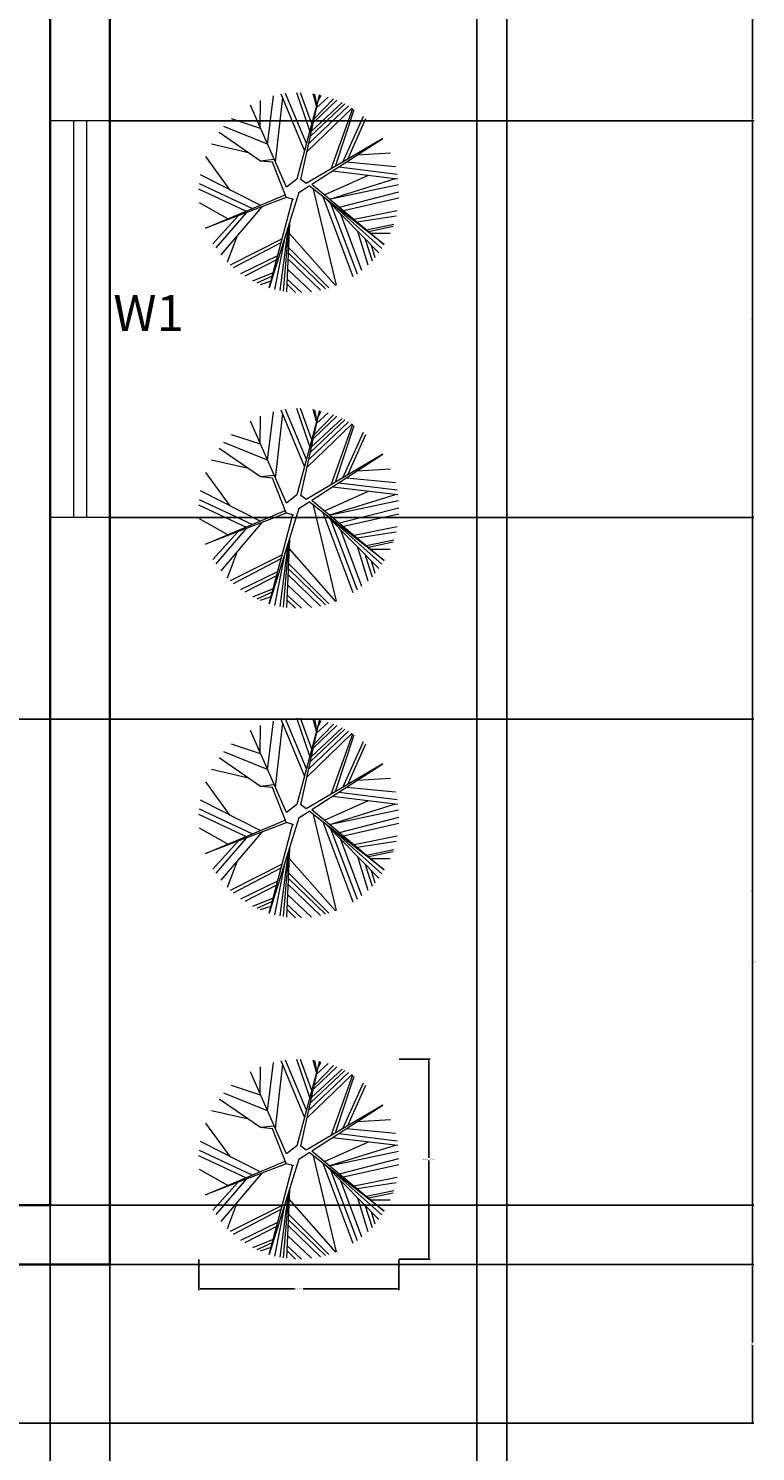
# Model space of a CAD drawing. Units: inches. Extents: x 503 to 1084, y -605 to 132.
# Tile 11 of 14: x 974 to 1084, y -392 to -177. Entities that reach past the tile are written whole.
import ezdxf

# ---------------------------------------------------------------- set-up
doc = ezdxf.new("R2010")
doc.units = ezdxf.units.IN
doc.header["$MEASUREMENT"] = 0
for name, color, linetype, lineweight in [('A-ANNO-DIMS', 7, 'Continuous', 18), ('A-ANNO-TEXT', 7, 'Continuous', 18), ('C-PROP', 1, 'Continuous', 25), ('wall', 1, 'Continuous', 35), ('wind', 5, 'Continuous', 18)]:
    doc.layers.add(name, color=color, linetype=linetype, lineweight=lineweight)
doc.layers.add('GRASS', color=90, linetype='Continuous', lineweight=13, transparency=0.7)
doc.styles.get("Standard").update_dxf_attribs({"font": 'arial.ttf'})
doc.dimstyles.get("Standard").update_dxf_attribs({"dimtxt": 0.18, "dimasz": 0.18, "dimexe": 0.18, "dimexo": 0.0625, "dimgap": 0.09, "dimtad": 0, "dimtih": 1, "dimtoh": 1, "dimdec": 1, "dimzin": 0, "dimdsep": 46, "dimlunit": 4, "dimtxsty": 'Standard', "dimcen": 0.09, "dimadec": 0, "dimazin": 0, "dimtfac": 1, "dimtdec": 1, "dimtofl": 0, "dimtmove": 0, "dimatfit": 3, "dimfxl": 1, "dimtolj": 1, "dimtzin": 0, "dimarcsym": 0})

# ---------------------------------------------------------------- blocks, each defined once
blk = doc.blocks.new('A$C4FA53466')
at = {"color": 0}
for p, q in [((0.91, 1.328), (0.802, 1.64)), ((0.925, 1.384), (0.834, 1.64)), ((0.717, 0.864), (0.422, 1.538)), ((0.501, 1.356), (0.505, 1.578)), ((0.563, 1.216), (0.612, 1.614)), ((0.627, 1.07), (0.687, 1.601)), ((0.867, 1.166), (0.675, 1.628)), ((0.882, 1.223), (0.709, 1.633)), ((0.988, 1.623), (0.804, 0.931)), ((0.836, 0.927), (0.988, 1.623)), ((0.901, 1.223), (1.228, 1.532)), ((0.914, 1.283), (1.197, 1.549)), ((0.922, 1.323), (1.176, 1.559)), ((0.964, 1.534), (0.938, 1.632)), ((0.938, 1.393), (1.132, 1.579)), ((0.945, 1.425), (1.104, 1.59)), ((0.967, 1.545), (0.952, 1.63)), ((0.965, 1.517), (1.059, 1.605)), ((0.974, 1.559), (1.002, 1.62)), ((0.505, 1.347), (0.266, 1.426)), ((0.887, 1.159), (1.256, 1.515)), ((1.085, 1.015), (1.262, 1.512)), ((1.121, 1.036), (1.274, 1.503)), ((1.18, 1.071), (1.349, 1.447)), ((1.222, 1.096), (1.37, 1.428)), ((0.506, 1.079), (0.165, 1.314)), ((0.562, 1.217), (0.205, 1.363)), ((0.406, 1.148), (0.102, 1.217)), ((1.509, 1.265), (0.879, 0.894)), ((0.926, 0.889), (1.509, 1.265)), ((0.255, 0.841), (0.055, 1.116)), ((0.614, 1.092), (0.506, 1.079)), ((0.604, 1.069), (0.506, 1.079)), ((0.715, 0.784), (0.604, 1.069)), ((1.211, 1.073), (1.612, 1.034)), ((1.3, 1.13), (1.573, 1.147)), ((0.501, 0.716), (0.012, 0.965)), ((1.03, 0.802), (1.392, 0.963)), ((1.073, 0.767), (1.614, 0.936)), ((1.097, 0.999), (1.632, 0.934)), ((1.148, 1.032), (1.626, 0.972)), ((0.384, 0.667), (0, 0.848)), ((0.436, 0.689), (0.003, 0.892)), ((0.82, 0.82), (0.575, 0.037)), ((0.804, 0.931), (0.717, 0.864)), ((0.82, 0.82), (0.904, 0.875)), ((0.879, 0.894), (0.836, 0.927)), ((1.521, 0.394), (0.904, 0.875)), ((0.926, 0.889), (1.521, 0.394)), ((0.938, 0.848), (1.126, 0.059)), ((1.081, 0.769), (1.638, 0.886)), ((1.153, 0.701), (1.64, 0.826)), ((0.237, 0.605), (0.004, 0.735)), ((0.053, 0.528), (0.708, 0.803)), ((0.716, 0.781), (0.053, 0.528)), ((0.516, 0.704), (0.179, 0.309)), ((0.575, 0.037), (0.769, 0.772)), ((0.715, 0.784), (0.775, 0.767)), ((1.016, 0.788), (1.263, 0.13)), ((1.04, 0.769), (1.475, 0.326)), ((1.06, 0.754), (1.5, 0.362)), ((1.083, 0.725), (1.298, 0.153)), ((1.185, 0.674), (1.639, 0.776)), ((0.321, 0.63), (0.115, 0.4)), ((0.387, 0.655), (0.137, 0.366)), ((1.161, 0.646), (1.335, 0.182)), ((1.273, 0.601), (1.627, 0.672)), ((1.298, 0.58), (1.618, 0.629)), ((0.732, 0.539), (0.664, 0.015)), ((0.737, 0.554), (0.691, 0.01)), ((0.744, 0.569), (0.717, 0.006)), ((0.74, 0.488), (1.121, 0.057)), ((1.301, 0.503), (1.386, 0.227)), ((1.376, 0.515), (1.599, 0.562)), ((1.392, 0.502), (1.593, 0.545)), ((1.412, 0.486), (1.569, 0.486)), ((0.313, 0.466), (0.232, 0.248)), ((0.682, 0.44), (0.255, 0.225)), ((0.673, 0.407), (0.281, 0.201)), ((0.701, 0.44), (0.621, 0.024)), ((0.735, 0.369), (1.067, 0.038)), ((1.365, 0.438), (1.42, 0.26)), ((1.413, 0.39), (1.444, 0.288)), ((0.645, 0.301), (0.342, 0.153)), ((0.636, 0.267), (0.375, 0.133)), ((0.73, 0.277), (0.998, 0.019)), ((0.733, 0.326), (1.037, 0.029)), ((0.608, 0.161), (0.439, 0.093)), ((0.6, 0.133), (0.475, 0.076)), ((0.726, 0.192), (0.924, 0.006)), ((0.59, 0.094), (0.501, 0.064)), ((0.72, 0.07), (0.793, 0)), ((0.722, 0.111), (0.842, 0))]:
    blk.add_line(p, q, dxfattribs=at)
blk = doc.blocks.new('*D20')
at = {"layer": 'A-ANNO-DIMS', "color": 0, "lineweight": -2, "transparency": 16777216}
for p, q in [((1029.85, -332.77), (1034.5, -332.77)), ((1034.32, -332.95), (1034.32, -347.69)), ((1034.32, -362.8), (1034.32, -348.06)), ((1029.85, -362.98), (1034.5, -362.98))]:
    blk.add_line(p, q, dxfattribs=at)
at = {"layer": 'A-ANNO-DIMS', "color": 0, "transparency": 16777216}
for points in [[(1034.29, -332.95), (1034.35, -332.95), (1034.32, -332.77)], [(1034.29, -362.8), (1034.35, -362.8), (1034.32, -362.98)]]:
    blk.add_solid(points, dxfattribs=at)
at = {"layer": 'Defpoints', "color": 0, "transparency": 16777216}
for p in [(1029.79, -332.77), (1034.32, -332.77), (1029.79, -362.98)]:
    blk.add_point(p, dxfattribs=at)
at = {"layer": 'A-ANNO-DIMS', "color": 0, "transparency": 16777216, "insert": (1034.32, -347.88), "char_height": 0.18, "attachment_point": 5}
blk.add_mtext('\\A1;SHRUB 2\'-6" TYP.', dxfattribs=at)
blk = doc.blocks.new('*D21')
at = {"layer": 'A-ANNO-DIMS', "color": 0, "lineweight": -2, "transparency": 16777216}
for p, q in [((999.58, -363.05), (999.58, -367.69)), ((1029.79, -363.05), (1029.79, -367.69)), ((999.76, -367.51), (1014.04, -367.51)), ((1029.61, -367.51), (1015.32, -367.51))]:
    blk.add_line(p, q, dxfattribs=at)
at = {"layer": 'A-ANNO-DIMS', "color": 0, "transparency": 16777216}
for points in [[(999.76, -367.48), (999.76, -367.54), (999.58, -367.51)], [(1029.61, -367.48), (1029.61, -367.54), (1029.79, -367.51)]]:
    blk.add_solid(points, dxfattribs=at)
at = {"layer": 'Defpoints', "color": 0, "transparency": 16777216}
for p in [(999.58, -362.98), (1029.79, -362.98), (1029.79, -367.51)]:
    blk.add_point(p, dxfattribs=at)
at = {"layer": 'A-ANNO-DIMS', "color": 0, "transparency": 16777216, "insert": (1014.68, -367.51), "char_height": 0.18, "attachment_point": 5}
blk.add_mtext('\\A1;2\'-6" TYP.', dxfattribs=at)
blk = doc.blocks.new('*D42')
at = {"layer": 'A-ANNO-DIMS', "color": 0, "lineweight": -2, "transparency": 16777216}
for p, q in [((986.15, -17.82), (1083.42, -17.82)), ((1083.24, -18), (1083.24, -190.63)), ((1083.24, -363.64), (1083.24, -191)), ((986.15, -363.82), (1083.42, -363.82))]:
    blk.add_line(p, q, dxfattribs=at)
at = {"layer": 'A-ANNO-DIMS', "color": 0, "transparency": 16777216}
for points in [[(1083.21, -18), (1083.27, -18), (1083.24, -17.82)], [(1083.21, -363.64), (1083.27, -363.64), (1083.24, -363.82)]]:
    blk.add_solid(points, dxfattribs=at)
at = {"layer": 'Defpoints', "color": 0, "transparency": 16777216}
for p in [(986.09, -17.82), (1083.24, -17.82), (986.09, -363.82)]:
    blk.add_point(p, dxfattribs=at)
at = {"layer": 'A-ANNO-DIMS', "color": 0, "transparency": 16777216, "insert": (1083.24, -190.82), "char_height": 0.18, "attachment_point": 5}
blk.add_mtext('\\A1;28\'-10"', dxfattribs=at)
blk = doc.blocks.new('*D43')
at = {"layer": 'A-ANNO-DIMS', "color": 0, "lineweight": -2, "transparency": 16777216}
for p, q in [((986.15, -190.82), (1083.42, -190.82)), ((1083.24, -191), (1083.24, -220.63)), ((1083.24, -250.64), (1083.24, -221)), ((986.15, -250.82), (1083.42, -250.82))]:
    blk.add_line(p, q, dxfattribs=at)
at = {"layer": 'A-ANNO-DIMS', "color": 0, "transparency": 16777216}
for points in [[(1083.21, -191), (1083.27, -191), (1083.24, -190.82)], [(1083.21, -250.64), (1083.27, -250.64), (1083.24, -250.82)]]:
    blk.add_solid(points, dxfattribs=at)
at = {"layer": 'Defpoints', "color": 0, "transparency": 16777216}
for p in [(986.09, -190.82), (986.09, -250.82), (1083.24, -250.82)]:
    blk.add_point(p, dxfattribs=at)
at = {"layer": 'A-ANNO-DIMS', "color": 0, "transparency": 16777216, "insert": (1083.24, -220.82), "char_height": 0.18, "attachment_point": 5}
blk.add_mtext('\\A1;5\'-0"', dxfattribs=at)
blk = doc.blocks.new('*D44')
at = {"layer": 'A-ANNO-DIMS', "color": 0, "lineweight": -2, "transparency": 16777216}
for p, q in [((986.15, -250.82), (1083.42, -250.82)), ((1083.24, -251), (1083.24, -307.13)), ((1083.24, -363.64), (1083.24, -307.5)), ((986.15, -363.82), (1083.42, -363.82))]:
    blk.add_line(p, q, dxfattribs=at)
at = {"layer": 'A-ANNO-DIMS', "color": 0, "transparency": 16777216}
for points in [[(1083.21, -251), (1083.27, -251), (1083.24, -250.82)], [(1083.21, -363.64), (1083.27, -363.64), (1083.24, -363.82)]]:
    blk.add_solid(points, dxfattribs=at)
at = {"layer": 'Defpoints', "color": 0, "transparency": 16777216}
for p in [(986.09, -250.82), (986.09, -363.82), (1083.24, -363.82)]:
    blk.add_point(p, dxfattribs=at)
at = {"layer": 'A-ANNO-DIMS', "color": 0, "transparency": 16777216, "insert": (1083.24, -307.32), "char_height": 0.18, "attachment_point": 5}
blk.add_mtext('\\A1;9\'-5"', dxfattribs=at)
blk = doc.blocks.new('*D47')
at = {"layer": 'A-ANNO-DIMS', "color": 0, "lineweight": -2, "transparency": 16777216}
for p, q in [((916.09, -363.88), (916.09, -583.15)), ((986.09, -363.88), (986.09, -583.15)), ((916.27, -582.97), (950.69, -582.97)), ((985.91, -582.97), (951.49, -582.97))]:
    blk.add_line(p, q, dxfattribs=at)
at = {"layer": 'A-ANNO-DIMS', "color": 0, "transparency": 16777216}
for points in [[(916.27, -582.94), (916.27, -583), (916.09, -582.97)], [(985.91, -582.94), (985.91, -583), (986.09, -582.97)]]:
    blk.add_solid(points, dxfattribs=at)
at = {"layer": 'Defpoints', "color": 0, "transparency": 16777216}
for p in [(916.09, -363.82), (986.09, -363.82), (986.09, -582.97)]:
    blk.add_point(p, dxfattribs=at)
at = {"layer": 'A-ANNO-DIMS', "color": 0, "transparency": 16777216, "insert": (951.09, -582.97), "char_height": 0.18, "attachment_point": 5}
blk.add_mtext('\\A1;5\'-10"', dxfattribs=at)
blk = doc.blocks.new('*D63')
at = {"layer": 'A-ANNO-DIMS', "color": 0, "lineweight": -2, "transparency": 16777216}
for p, q in [((783.15, -281.32), (1083.42, -281.32)), ((1083.24, -281.5), (1083.24, -317.88)), ((1083.24, -354.64), (1083.24, -318.25)), ((783.15, -354.82), (1083.42, -354.82))]:
    blk.add_line(p, q, dxfattribs=at)
at = {"layer": 'A-ANNO-DIMS', "color": 0, "transparency": 16777216}
for points in [[(1083.21, -281.5), (1083.27, -281.5), (1083.24, -281.32)], [(1083.21, -354.64), (1083.27, -354.64), (1083.24, -354.82)]]:
    blk.add_solid(points, dxfattribs=at)
at = {"layer": 'Defpoints', "color": 0, "transparency": 16777216}
for p in [(783.09, -281.32), (783.09, -354.82), (1083.24, -354.82)]:
    blk.add_point(p, dxfattribs=at)
at = {"layer": 'A-ANNO-DIMS', "color": 0, "transparency": 16777216, "insert": (1083.24, -318.07), "char_height": 0.18, "attachment_point": 5}
blk.add_mtext('\\A1;6\'-1 1/2"', dxfattribs=at)
blk = doc.blocks.new('*D64')
at = {"layer": 'A-ANNO-DIMS', "color": 0, "lineweight": -2, "transparency": 16777216}
for p, q in [((938.09, -162.88), (938.09, -583.15)), ((977.09, -162.88), (977.09, -583.15)), ((938.27, -582.97), (957.26, -582.97)), ((976.91, -582.97), (957.92, -582.97))]:
    blk.add_line(p, q, dxfattribs=at)
at = {"layer": 'A-ANNO-DIMS', "color": 0, "transparency": 16777216}
for points in [[(938.27, -582.94), (938.27, -583), (938.09, -582.97)], [(976.91, -582.94), (976.91, -583), (977.09, -582.97)]]:
    blk.add_solid(points, dxfattribs=at)
at = {"layer": 'Defpoints', "color": 0, "transparency": 16777216}
for p in [(938.09, -162.82), (977.09, -162.82), (977.09, -582.97)]:
    blk.add_point(p, dxfattribs=at)
at = {"layer": 'A-ANNO-DIMS', "color": 0, "transparency": 16777216, "insert": (957.59, -582.97), "char_height": 0.18, "attachment_point": 5}
blk.add_mtext('\\A1;3\'-3"', dxfattribs=at)
blk = doc.blocks.new('*D67')
at = {"layer": 'A-ANNO-DIMS', "color": 0, "lineweight": -2, "transparency": 16777216}
for p, q in [((921.26, -363.82), (1083.42, -363.82)), ((1083.24, -364), (1083.24, -375.63)), ((1083.24, -387.64), (1083.24, -376)), ((921.26, -387.82), (1083.42, -387.82))]:
    blk.add_line(p, q, dxfattribs=at)
at = {"layer": 'A-ANNO-DIMS', "color": 0, "transparency": 16777216}
for points in [[(1083.21, -364), (1083.27, -364), (1083.24, -363.82)], [(1083.21, -387.64), (1083.27, -387.64), (1083.24, -387.82)]]:
    blk.add_solid(points, dxfattribs=at)
at = {"layer": 'Defpoints', "color": 0, "transparency": 16777216}
for p in [(921.2, -363.82), (1083.24, -363.82), (921.2, -387.82)]:
    blk.add_point(p, dxfattribs=at)
at = {"layer": 'A-ANNO-DIMS', "color": 0, "transparency": 16777216, "insert": (1083.24, -375.82), "char_height": 0.18, "attachment_point": 5}
blk.add_mtext('\\A1;2\'-0"', dxfattribs=at)

msp = doc.modelspace()

# ---------------------------------------------------------------- linework, layer by layer
at = {"layer": 'C-PROP'}
for p, q in [((1046.09, 6.18), (1046.09, -545.82)), ((1041.59, -541.32), (1041.59, 1.68))]:
    msp.add_line(p, q, dxfattribs=at)
at = {"layer": 'wall'}
for p, q in [((986.09, -17.82), (986.09, -363.82)), ((977.09, -162.82), (977.09, -354.82)), ((916.09, -354.82), (977.09, -354.82)), ((916.09, -363.82), (986.09, -363.82))]:
    msp.add_line(p, q, dxfattribs=at)
at = {"layer": 'wind'}
for p, q in [((986.09, -190.82), (977.09, -190.82)), ((980.59, -190.82), (980.59, -250.82)), ((982.59, -190.82), (982.59, -250.82)), ((986.09, -250.82), (977.09, -250.82))]:
    msp.add_line(p, q, dxfattribs=at)

# ---------------------------------------------------------------- block references
at = {"layer": 'GRASS', "xscale": 18.41745235960633, "yscale": 18.41745235960633, "zscale": 18.41745235960633}
for p in [(999.58, -216.77), (999.58, -264.55), (999.58, -311.36), (999.58, -362.98)]:
    msp.add_blockref('A$C4FA53466', p, dxfattribs=at)

# ---------------------------------------------------------------- texts
at = {"layer": 'A-ANNO-TEXT'}
msp.add_text('W1', height=5.444, dxfattribs=at).set_placement((986.64, -222.61))

# ---------------------------------------------------------------- dimensions: what is measured, and where the dimension line sits
at = {"layer": 'A-ANNO-DIMS'}
for base, p1, p2, picture, middle in [((1083.24, -17.82), (986.09, -363.82), (986.09, -17.82), '*D42', (1083.24, -190.82)), ((1083.24, -250.82), (986.09, -190.82), (986.09, -250.82), '*D43', (1083.24, -220.82)), ((1083.24, -363.82), (986.09, -250.82), (986.09, -363.82), '*D44', (1083.24, -307.32)), ((1083.24, -354.82), (783.09, -281.32), (783.09, -354.82), '*D63', (1083.24, -318.07)), ((1083.24, -363.82), (921.2, -387.82), (921.2, -363.82), '*D67', (1083.24, -375.82))]:
    dim = msp.add_linear_dim(base=base, p1=p1, p2=p2, angle=90, dimstyle='Standard', override={"dimdec": 1, "dimlfac": 1, "dimrnd": 0, "dimzin": 1, "dimdsep": 46, "dimlunit": 4, "dimfrac": 2}, dxfattribs=at)
    dim.commit()
    dim.dimension.update_dxf_attribs({"geometry": picture, "text_midpoint": middle})
for base, p1, p2, picture, middle in [((977.09, -582.97), (938.09, -162.82), (977.09, -162.82), '*D64', (957.59, -582.97)), ((986.09, -582.97), (916.09, -363.82), (986.09, -363.82), '*D47', (951.09, -582.97))]:
    dim = msp.add_linear_dim(base=base, p1=p1, p2=p2, dimstyle='Standard', override={"dimdec": 1, "dimlfac": 1, "dimrnd": 0, "dimzin": 1, "dimdsep": 46, "dimlunit": 4, "dimfrac": 2}, dxfattribs=at)
    dim.commit()
    dim.dimension.update_dxf_attribs({"geometry": picture, "text_midpoint": middle})
dim = msp.add_linear_dim(base=(1034.32, -332.77), p1=(1029.79, -362.98), p2=(1029.79, -332.77), angle=90, text='SHRUB <> TYP.', dimstyle='Standard', override={"dimdec": 1, "dimlfac": 1, "dimrnd": 0, "dimzin": 1, "dimdsep": 46, "dimlunit": 4, "dimfrac": 2}, dxfattribs=at)
dim.commit()
dim.dimension.update_dxf_attribs({"geometry": '*D20', "text_midpoint": (1034.32, -347.88)})
dim = msp.add_linear_dim(base=(1029.79, -367.51), p1=(999.58, -362.98), p2=(1029.79, -362.98), text='<> TYP.', dimstyle='Standard', override={"dimdec": 1, "dimlfac": 1, "dimrnd": 0, "dimzin": 1, "dimdsep": 46, "dimlunit": 4, "dimfrac": 2}, dxfattribs=at)
dim.commit()
dim.dimension.update_dxf_attribs({"geometry": '*D21', "text_midpoint": (1014.68, -367.51)})

doc.saveas('drawing.dxf')
